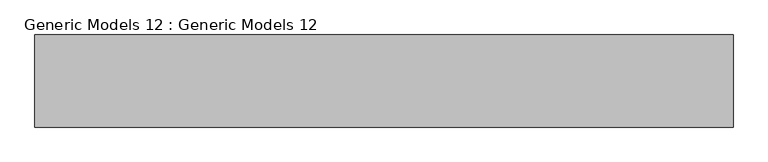
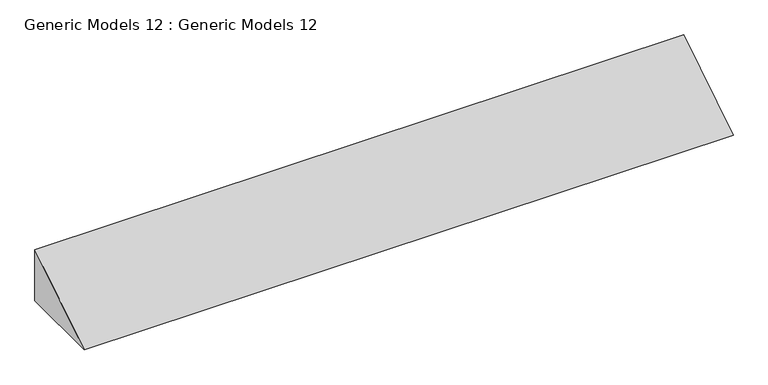
"""IFC4 building model written with IfcOpenShell, lengths in millimetres: proxy geometry, Generic Models 12 : Generic Models 12."""

from ifc_helpers import new_model, si_unit, frame, origin, place, context, project, spatial, polyline, outline, extrude, source, transform, mapped, element, save


def generic_models_12_generic_models_12_89349366(model_context):
    return source(origin(), model_context, "Body", "SweptSolid", [
        extrude(outline(polyline([(-14633.8396616, 0.0), (-15116.4396616, 0.0), (-14633.8396616, 304.8), (-14633.8396616, 0.0)])), frame((-11570.0008118, 0.0, 0.0), z_axis=(1.0, 0.0, 0.0), x_axis=(0.0, 1.0, 0.0)), (0.0, 0.0, 1.0), 3657.6875254),
    ])


if __name__ == "__main__":
    model = new_model("IFC4")
    model_context = context("Model", 3, world=origin())
    ifc_project = project(units=[si_unit("LENGTHUNIT", "METRE", prefix="MILLI")], contexts=[model_context])
    site = spatial("IfcSite", under=ifc_project)
    building = spatial("IfcBuilding", under=site)
    placement = place(None, origin())
    generic_models_12_generic_models_12_shape = generic_models_12_generic_models_12_89349366(model_context)
    element("IfcBuildingElementProxy", 1, Name="Generic Models 12 : Generic Models 12", ObjectType="Generic Models 12 : Generic Models 12", at=placement, inside=building, context=model_context, shape_type="MappedRepresentation", body=[
        mapped(generic_models_12_generic_models_12_shape, transform((0.0, 0.0, 0.0), x_axis=(1.0, 0.0, 0.0), y_axis=(0.0, 1.0, 0.0), z_axis=(0.0, 0.0, 1.0))),
    ])
    save(model, "model.ifc")

# Revit data of these elements
# Element 1 (IfcBuildingElementProxy, "Generic Models 12 : Generic Models 12")
#   Materials on its faces: "Concrete, Cast-in-Place gray"
# Materials
#   "Concrete, Cast-in-Place gray": class "Concrete", colour RGB 192 192 192, transparency 0, Description = "Cast-in-place concrete", Cost = 0
